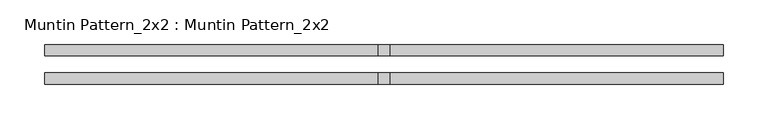
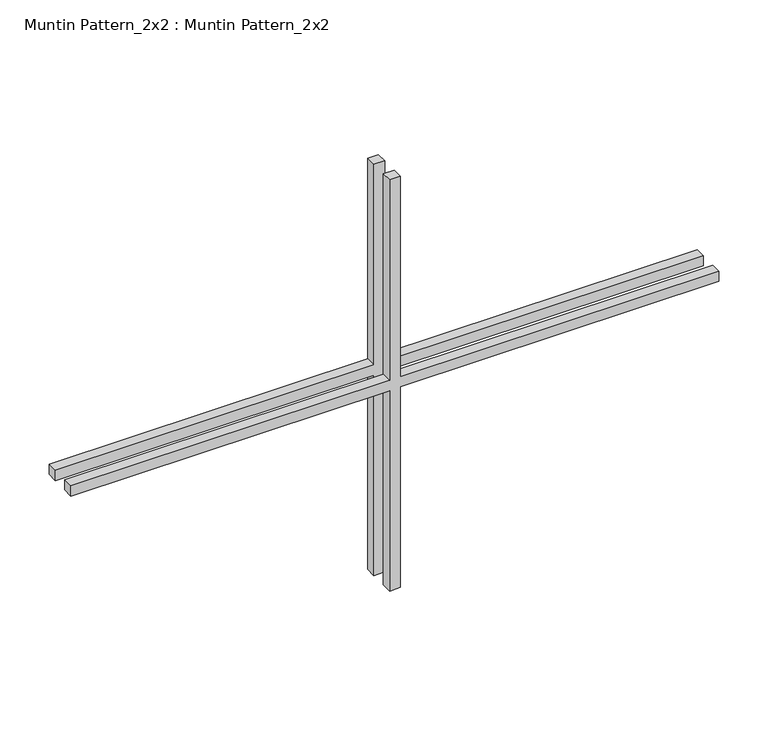
"""IFC4 building model written with IfcOpenShell, lengths in millimetres: proxy geometry, Muntin Pattern_2x2 : Muntin Pattern_2x2."""

from ifc_helpers import new_model, si_unit, frame, origin, place, context, project, spatial, polyline, outline, extrude, source, transform, mapped, element, save


def muntin_pattern_2x2_muntin_pattern_2x2_f2410a90(model_context):
    return source(origin(), model_context, "Body", "SweptSolid", [
        extrude(outline(polyline([(261.9375, -6.35), (261.9375, -381.0), (249.2375, -381.0), (249.2375, -6.35), (0.0, -6.35), (0.0, 6.35), (249.2375, 6.35), (249.2375, 381.0), (261.9375, 381.0), (261.9375, 6.35), (511.175, 6.35), (511.175, -6.35), (261.9375, -6.35)])), frame((0.0, 9.525, 0.0), z_axis=(0.0, 1.0, 0.0), x_axis=(0.0, 0.0, 1.0)), (0.0, 0.0, 1.0), 12.7),
        extrude(outline(polyline([(261.9375, -6.35), (261.9375, -381.0), (249.2375, -381.0), (249.2375, -6.35), (0.0, -6.35), (0.0, 6.35), (249.2375, 6.35), (249.2375, 381.0), (261.9375, 381.0), (261.9375, 6.35), (511.175, 6.35), (511.175, -6.35), (261.9375, -6.35)])), frame((0.0, -22.225, 0.0), z_axis=(0.0, 1.0, 0.0), x_axis=(0.0, 0.0, 1.0)), (0.0, 0.0, 1.0), 12.7),
    ])


if __name__ == "__main__":
    model = new_model("IFC4")
    model_context = context("Model", 3, world=origin())
    ifc_project = project(units=[si_unit("LENGTHUNIT", "METRE", prefix="MILLI")], contexts=[model_context])
    site = spatial("IfcSite", under=ifc_project)
    building = spatial("IfcBuilding", under=site)
    placement = place(None, origin())
    muntin_pattern_2x2_muntin_pattern_2x2_shape = muntin_pattern_2x2_muntin_pattern_2x2_f2410a90(model_context)
    element("IfcBuildingElementProxy", 1, Name="Muntin Pattern_2x2 : Muntin Pattern_2x2", ObjectType="Muntin Pattern_2x2 : Muntin Pattern_2x2", at=placement, inside=building, context=model_context, shape_type="MappedRepresentation", body=[
        mapped(muntin_pattern_2x2_muntin_pattern_2x2_shape, transform((0.0, 0.0, 0.0), x_axis=(1.0, 0.0, 0.0), y_axis=(0.0, 1.0, 0.0), z_axis=(0.0, 0.0, 1.0))),
    ])
    save(model, "model.ifc")

# Revit data of these elements
# Type "Muntin Pattern_2x2 : Muntin Pattern_2x2"
#   Width [instance default] = 4' - 0"
#   Thickness = 0' - 0 1/2"
#   Height [instance default] = 4' - 0"
#   Distance = 0' - 0 3/4"
#   Interior Material [instance default] = none
#   Exterior Material [instance default] = none
#   Default Elevation = 0
# Element 1 (IfcBuildingElementProxy, "Muntin Pattern_2x2 : Muntin Pattern_2x2")
#   Width = 2' - 6"
#   Height = 1' - 8 1/8"
#   Interior Material = Wood - Stained
#   Exterior Material = Clad - White
#   Materials on its faces: "Clad - White", "Wood - Stained"
# Materials
#   "Clad - White": class "Wood", colour RGB 242 242 238, transparency 0, Cost = 0
#   "Wood - Stained": class "Wood", colour RGB 224 178 126, transparency 0, Cost = 0
